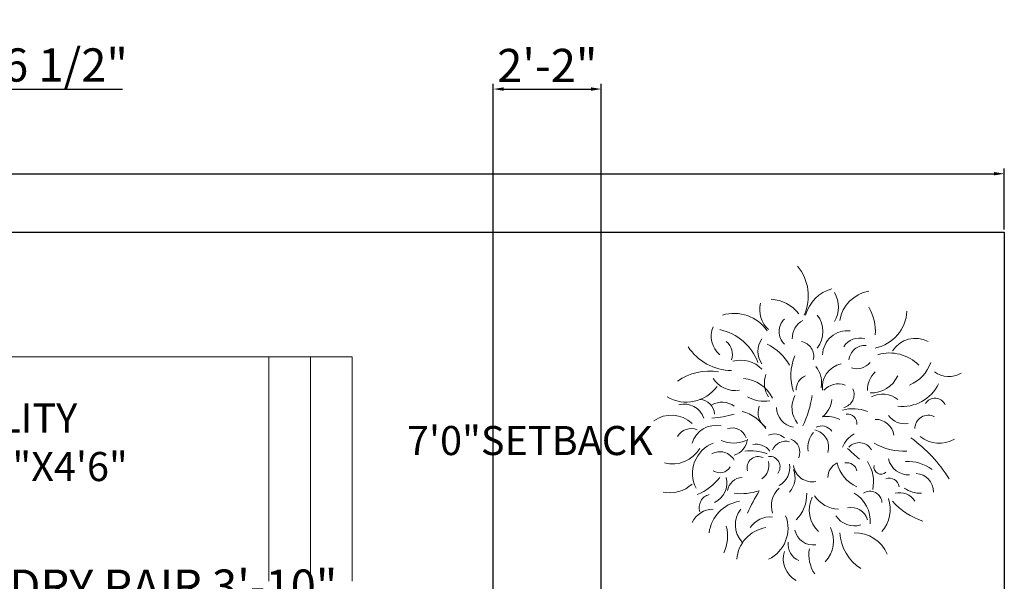
# Model space of a CAD drawing. Units: inches. Extents: x 3394 to 4794, y 965 to 1718.
# Tile 11 of 15: x 3704 to 3941, y 1583 to 1718. Entities that reach past the tile are written whole.
import ezdxf

# ---------------------------------------------------------------- set-up
doc = ezdxf.new("R2010")
doc.units = ezdxf.units.IN
for name, color, linetype, lineweight in [('A-ANNO-DIMS', 2, 'Continuous', 13), ('A-ANNO-TEXT', 7, 'Continuous', 18), ('A-AREA-IDEN', 7, 'Continuous', 18), ('A-FLOR', 7, 'Continuous', 18), ('A-FLOR-STRS', 7, 'Continuous', 18), ('C-PROP', 7, 'Continuous', 25), ('CAY', 94, 'Continuous', 13)]:
    doc.layers.add(name, color=color, linetype=linetype, lineweight=lineweight)
doc.styles.add('ATT', font='romans.shx')
doc.styles.get("Standard").update_dxf_attribs({"font": 'arial.ttf'})
doc.dimstyles.new('ISO-25', dxfattribs={"dimtxt": 8, "dimasz": 2.5, "dimexe": 1.25, "dimexo": 0.625, "dimtad": 1, "dimlunit": 3, "dimtxsty": 'Standard', "dimcen": 2.5, "dimadec": 0, "dimazin": 0, "dimtfac": 1, "dimtmove": 0, "dimatfit": 3, "dimfxl": 1, "dimarcsym": 0})

# ---------------------------------------------------------------- blocks, each defined once
blk = doc.blocks.new('12PPLT14')
at = {"color": 0, "linetype": 'ByBlock'}
for centre, radius, start, end in [((-0.1625, 0.4338), 0.1552, 335.4234, 39.9527), ((0.1087, 0.3325), 0.1308, 106.3737, 163.6865), ((-0.0015, 0.3959), 0.0956, 329.2952, 30.7048), ((0.216, 0.3316), 0.1193, 99.6686, 170.3916), ((-0.0808, 0.3868), 0.0897, 165.5676, 227.7978), ((-0.1402, 0.294), 0.1288, 38.2331, 86.4254), ((-0.2571, 0.2399), 0.1351, 34.2662, 106.816), ((-0.0514, 0.3138), 0.0928, 323.3029, 36.6971), ((0.0506, 0.3121), 0.1678, 356.7873, 29.9706), ((0.1909, 0.3893), 0.1338, 281.7312, 357.1257), ((-0.0467, 0.3138), 0.0589, 134.2792, 225.7208), ((0.0083, 0.2908), 0.0696, 119.3333, 181.2289), ((-0.2523, 0.2979), 0.0813, 157.2527, 229.5051), ((-0.3428, 0.1468), 0.1777, 20.6522, 77.761), ((0.1238, 0.2336), 0.083, 82.9962, 178.2659), ((-0.3207, 0.2361), 0.0583, 342.2672, 49.5918), ((-0.1032, 0.2472), 0.0733, 144.9004, 215.0996), ((-0.223, 0.1138), 0.1758, 29.5718, 63.8395), ((-0.0403, 0.2301), 0.0513, 346.7243, 78.6914), ((0.1649, 0.2288), 0.0631, 73.677, 147.4747), ((0.1827, 0.2139), 0.0534, 85.265, 175.2671), ((0.3529, 0.1986), 0.0923, 62.4899, 146.6083), ((-0.2631, 0.3606), 0.1778, 213.4024, 269.326), ((0.2662, 0.1039), 0.1379, 44.5227, 106.5076), ((-0.2335, 0.1217), 0.0961, 42.9815, 106.4777), ((0.103, 0.1659), 0.1687, 157.0616, 198.7007), ((0.1187, 0.1278), 0.0788, 101.6359, 188.4366), ((0.1561, 0.2471), 0.0582, 252.2434, 319.6792), ((0.2843, 0.2512), 0.1271, 292.7233, 340.8083), ((-0.3406, -0.0039), 0.1849, 80.336, 125.1387), ((-0.071, 0.1405), 0.0841, 159.833, 213.5727), ((-0.0525, 0.1406), 0.0902, 350.0819, 37.9622), ((0.2797, 0.1152), 0.0882, 134.2975, 179.349), ((0.4652, 0.2401), 0.0779, 232.4069, 301.8623), ((-0.2521, 0.2046), 0.0894, 212.7771, 278.7223), ((-0.2353, 0.0367), 0.1199, 26.1776, 85.1926), ((0.002, 0.1188), 0.05, 112.1748, 182.9374), ((0.094, 0.072), 0.0659, 70.3325, 137.7683), ((0.2042, 0.2053), 0.098, 267.7941, 335.7788), ((0.3092, 0.1973), 0.1353, 263.3454, 334.185), ((-0.4178, 0.2048), 0.1282, 239.7244, 324.0772), ((0.1017, 0.1024), 0.045, 282.8815, 24.0365), ((0.2424, 0.0217), 0.0815, 51.1397, 117.4271), ((-0.4247, -0.0009), 0.0706, 19.8329, 104.6003), ((-0.3739, 0.0341), 0.0511, 2.467, 87.4728), ((-0.2974, 0.0074), 0.0691, 53.5126, 119.7474), ((-0.1543, 0.2003), 0.1209, 241.5287, 278.4347), ((0.0228, 0.0586), 0.0851, 152.0419, 218.8274), ((-0.34, 0.1477), 0.3488, 334.29, 351.8885), ((-0.0111, 0.0925), 0.0832, 308.5351, 354.9136), ((0.4187, 0.0518), 0.0378, 24.3786, 147.9852), ((-0.3432, 0.3083), 0.2855, 272.3147, 287.7219), ((-0.2616, -0.0829), 0.132, 32.2356, 76.0319), ((-0.1183, 0.0408), 0.0581, 157.5609, 237.1128), ((-0.0447, 0.0607), 0.0698, 181.7454, 260.0237), ((0.1427, -0.0803), 0.1346, 68.7259, 105.2422), ((0.125, 0.0053), 0.0314, 351.8398, 98.1), ((-0.468, -0.0701), 0.1027, 47.2022, 124.8992), ((0.0563, -0.0634), 0.0921, 62.7918, 99.6978), ((0.2201, -0.0419), 0.0605, 6.851, 91.8869), ((0.3159, 0.0688), 0.0649, 214.6894, 281.6662), ((0.3966, -0.0128), 0.0455, 62.415, 179.5656), ((-0.4019, -0.0635), 0.0512, 65.2631, 151.643), ((-0.3178, -0.086), 0.0842, 78.2859, 162.9253), ((-0.2636, -0.0603), 0.0501, 19.5336, 107.2881), ((-0.1211, -0.079), 0.0486, 46.81, 114.2458), ((0.0687, -0.0762), 0.0776, 139.4669, 188.6741), ((0.0015, -0.0752), 0.0596, 343.1915, 77.687), ((0.0376, -0.0452), 0.0417, 34.8572, 117.0419), ((0.197, -0.1152), 0.0984, 120.3942, 155.6913), ((-0.2877, -0.1629), 0.109, 111.2663, 206.9249), ((-0.2585, 0.0428), 0.1041, 246.1369, 293.8631), ((-0.2726, -0.0426), 0.0609, 285.5398, 354.9083), ((-0.1835, -0.1238), 0.059, 37.3855, 100.4991), ((-0.0834, -0.1038), 0.0488, 74.167, 155.4291), ((-0.0828, -0.0921), 0.0473, 337.5706, 68.783), ((0.1639, -0.1068), 0.0471, 29.6516, 136.9148), ((0.3131, 0.1083), 0.1966, 239.6382, 273.343), ((0.055, -0.4368), 0.4844, 31.8508, 54.2708), ((0.4332, 0.0428), 0.1041, 231.8734, 299.32), ((-0.465, -0.0212), 0.1099, 256.1392, 328.2356), ((-0.3051, -0.1456), 0.0555, 28.564, 118.6243), ((-0.2031, -0.2618), 0.1748, 70.7416, 95.8247), ((0.3403, 0.1226), 0.295, 223.1416, 233.5315), ((-0.1751, -0.1446), 0.0382, 64.5989, 195.0715), ((-0.1983, -0.1346), 0.0584, 307.0043, 10.961), ((-0.1379, -0.1412), 0.0356, 321.496, 95.0552), ((-0.1367, -0.1434), 0.0675, 297.4603, 9.4578), ((0.1122, -0.1766), 0.0537, 114.9911, 180.121), ((0.2021, -0.1018), 0.1155, 193.035, 246.5169), ((0.1228, -0.1611), 0.0339, 11.252, 101.3122), ((0.0954, -0.19), 0.1169, 346.8331, 34.7134), ((0.3301, -0.0984), 0.0696, 193.4793, 272.7231), ((0.3295, -0.2531), 0.1299, 52.4116, 94.1568), ((-0.3049, -0.1199), 0.0412, 237.1862, 328.8294), ((-0.1261, -0.1768), 0.0743, 318.9446, 21.0601), ((0.0056, -0.1284), 0.0629, 187.6037, 281.9043), ((0.2371, -0.1417), 0.0239, 167.9887, 313.8509), ((0.3525, -0.2241), 0.0608, 358.6144, 87.0834), ((-0.4582, -0.0549), 0.1957, 293.3946, 321.4742), ((-0.3545, -0.1945), 0.0737, 295.4172, 13.937), ((-0.2272, -0.2284), 0.0518, 92.735, 171.8723), ((0.265, -0.2125), 0.0333, 8.0854, 109.9339), ((-0.4721, -0.1203), 0.1079, 257.3279, 313.213), ((-0.2342, -0.0362), 0.1951, 263.4737, 288.5568), ((0.4875, -0.6182), 0.7699, 148.9497, 155.3056), ((-0.0491, -0.2722), 0.0823, 133.2929, 197.2496), ((-0.1342, -0.2328), 0.1218, 315.1067, 1.332), ((0.0948, -0.3222), 0.106, 354.6407, 60.4156), ((0.2004, -0.2632), 0.04, 3.1298, 123.6919), ((0.3002, -0.2876), 0.0597, 31.279, 105.0766), ((0.3711, -0.1347), 0.0953, 234.4297, 271.3309), ((-0.3303, -0.2772), 0.044, 103.5534, 199.8954), ((-0.2197, -0.3768), 0.1216, 98.9327, 173.5652), ((0.0958, -0.2858), 0.1, 154.8808, 226.8679), ((0.0984, -0.1813), 0.1021, 214.3427, 267.4969), ((0.1534, -0.2836), 0.1149, 319.1908, 18.2125), ((0.4504, -0.1006), 0.2342, 221.7868, 251.9354), ((-0.3258, -0.3645), 0.0813, 91.0528, 153.0122), ((-0.1666, -0.3361), 0.0858, 141.9374, 222.639), ((0.137, -0.3342), 0.0567, 15.8404, 102.1789), ((-0.1356, -0.3909), 0.0814, 84.4526, 145.9961), ((-0.1912, -0.3476), 0.1157, 295.6702, 21.368), ((0.1487, -0.2627), 0.0766, 213.8932, 285.618), ((-0.4022, -0.3739), 0.1237, 333.1557, 15.4351), ((-0.1321, -0.4596), 0.1156, 98.8586, 176.1805), ((0.0095, -0.3403), 0.0634, 192.7121, 278.2146), ((-0.0287, -0.3897), 0.1058, 317.7735, 24.7522), ((0.2528, -0.3527), 0.1547, 183.8744, 237.3741), ((0.1506, -0.4799), 0.1168, 23.0406, 91.6662), ((-0.0165, -0.4023), 0.0586, 172.0702, 247.3677), ((-0.0081, -0.4497), 0.0833, 162.968, 241.4878), ((0.1108, -0.4364), 0.1161, 170.0959, 213.6572)]:
    blk.add_arc(centre, radius, start, end, dxfattribs=at)
at = {"color": 0, "linetype": 'ByBlock', "style": 'ATT'}
for tag, p, flags in [('ITEM', (-1.4111, -3.0457), 3), ('ROOM_NUMBER', (-1.4111, -4.379), 1)]:
    blk.add_attdef(tag, p, '', height=1, dxfattribs=dict(at, flags=flags))
blk = doc.blocks.new('*D30')
at = {"layer": 'A-ANNO-DIMS', "color": 0, "lineweight": -2, "transparency": 16777216}
for p, q in [((3427.74, 1667.31), (3427.74, 1682.01)), ((3430.24, 1680.76), (3938.24, 1680.76)), ((3940.74, 1667.31), (3940.74, 1682.01))]:
    blk.add_line(p, q, dxfattribs=at)
at = {"layer": 'A-ANNO-DIMS', "color": 0, "transparency": 16777216}
for points in [[(3430.24, 1681.18), (3430.24, 1680.35), (3427.74, 1680.76)], [(3938.24, 1681.18), (3938.24, 1680.35), (3940.74, 1680.76)]]:
    blk.add_solid(points, dxfattribs=at)
at = {"layer": 'Defpoints', "color": 0, "transparency": 16777216}
for p in [(3940.74, 1680.76), (3427.74, 1666.68), (3940.74, 1666.68)]:
    blk.add_point(p, dxfattribs=at)
at = {"layer": 'A-ANNO-DIMS', "color": 0, "transparency": 16777216, "insert": (3684.24, 1685.47), "char_height": 8, "attachment_point": 5}
blk.add_mtext('42\'-9"', dxfattribs=at)
blk = doc.blocks.new('*D92')
at = {"layer": 'A-ANNO-DIMS', "color": 0, "lineweight": -2, "transparency": 16777216}
for p, q in [((3620.92, 1582.06), (3620.92, 1574.52)), ((3667.02, 1582.06), (3667.02, 1574.52)), ((3623.42, 1575.77), (3664.52, 1575.77)), ((3667.02, 1575.77), (3783.6, 1575.77))]:
    blk.add_line(p, q, dxfattribs=at)
at = {"layer": 'A-ANNO-DIMS', "color": 0, "transparency": 16777216}
for points in [[(3623.42, 1576.18), (3623.42, 1575.35), (3620.92, 1575.77)], [(3664.52, 1576.18), (3664.52, 1575.35), (3667.02, 1575.77)]]:
    blk.add_solid(points, dxfattribs=at)
at = {"layer": 'Defpoints', "color": 0, "transparency": 16777216}
for p in [(3620.92, 1582.68), (3667.02, 1582.68), (3667.02, 1575.77)]:
    blk.add_point(p, dxfattribs=at)
at = {"layer": 'A-ANNO-DIMS', "color": 0, "transparency": 16777216, "insert": (3726.56, 1580.48), "char_height": 8, "attachment_point": 5}
blk.add_mtext('LAUNDRY PAIR 3\'-10"', dxfattribs=at)
blk = doc.blocks.new('*D124')
at = {"layer": 'A-ANNO-DIMS', "color": 0, "lineweight": -2, "transparency": 16777216}
for p, q in [((3667.02, 1583.31), (3667.02, 1702.38)), ((3685.62, 1583.31), (3685.62, 1702.38)), ((3669.52, 1701.13), (3683.12, 1701.13)), ((3685.62, 1701.13), (3728.52, 1701.13))]:
    blk.add_line(p, q, dxfattribs=at)
at = {"layer": 'A-ANNO-DIMS', "color": 0, "transparency": 16777216}
for points in [[(3669.52, 1701.55), (3669.52, 1700.72), (3667.02, 1701.13)], [(3683.12, 1701.55), (3683.12, 1700.72), (3685.62, 1701.13)]]:
    blk.add_solid(points, dxfattribs=at)
at = {"layer": 'Defpoints', "color": 0, "transparency": 16777216}
for p in [(3685.62, 1701.13), (3667.02, 1582.68), (3685.62, 1582.68)]:
    blk.add_point(p, dxfattribs=at)
at = {"layer": 'A-ANNO-DIMS', "color": 0, "transparency": 16777216, "insert": (3708.32, 1705.89), "char_height": 8, "attachment_point": 5}
blk.add_mtext('1\'-6 1/2"', dxfattribs=at)
blk = doc.blocks.new('*D126')
at = {"layer": 'A-ANNO-DIMS', "color": 0, "lineweight": -2, "transparency": 16777216}
for p, q in [((3817.74, 1382.31), (3817.74, 1702.38)), ((3843.73, 1380.81), (3843.73, 1702.38)), ((3820.24, 1701.13), (3841.23, 1701.13))]:
    blk.add_line(p, q, dxfattribs=at)
at = {"layer": 'A-ANNO-DIMS', "color": 0, "transparency": 16777216}
for points in [[(3820.24, 1701.55), (3820.24, 1700.72), (3817.74, 1701.13)], [(3841.23, 1701.55), (3841.23, 1700.72), (3843.73, 1701.13)]]:
    blk.add_solid(points, dxfattribs=at)
at = {"layer": 'Defpoints', "color": 0, "transparency": 16777216}
for p in [(3843.73, 1701.13), (3817.74, 1381.68), (3843.73, 1380.18)]:
    blk.add_point(p, dxfattribs=at)
at = {"layer": 'A-ANNO-DIMS', "color": 0, "transparency": 16777216, "insert": (3830.74, 1705.77), "char_height": 8, "attachment_point": 5}
blk.add_mtext('2\'-2"', dxfattribs=at)

msp = doc.modelspace()

# ---------------------------------------------------------------- linework, layer by layer
at = {"layer": 'A-FLOR'}
msp.add_line((3783.745, 1636.682), (3604.745, 1636.682), dxfattribs=at)
at = {"layer": 'A-FLOR-STRS'}
for p, q in [((3763.745, 1582.682), (3763.745, 1636.682)), ((3773.745, 1582.682), (3773.745, 1636.682)), ((3783.745, 1582.682), (3783.745, 1636.682))]:
    msp.add_line(p, q, dxfattribs=at)
at = {"layer": 'C-PROP'}
for p, q in [((3427.745, 1666.682), (3940.745, 1666.682)), ((3940.745, 1666.682), (3940.745, 1057.682))]:
    msp.add_line(p, q, dxfattribs=at)

# ---------------------------------------------------------------- block references
at = {"layer": 'CAY', "xscale": 71.57720376410516, "yscale": 71.57720376410516, "zscale": 71.57720376410516}
msp.add_blockref('12PPLT14', (3894.085, 1620.317), dxfattribs=at)

# ---------------------------------------------------------------- texts
at = {"layer": 'A-ANNO-TEXT', "insert": (3796.969, 1620.056), "char_height": 7, "attachment_point": 1}
msp.add_mtext_dynamic_manual_height_columns('{\\fTimes New Roman|b0|i0|c0|p18;7\'0"SETBACK}', width=61.05572, gutter_width=12.5, heights=[0], dxfattribs=at)
at = {"layer": 'A-AREA-IDEN', "insert": (3683.427, 1625.469), "char_height": 7, "attachment_point": 1}
msp.add_mtext_dynamic_manual_height_columns('{\\fTimes New Roman|b0|i0|c0|p18;UTILITY\\P13\'3"X4\'6"}', width=61.05572, gutter_width=12.5, heights=[0], dxfattribs=at)

# ---------------------------------------------------------------- dimensions: what is measured, and where the dimension line sits
at = {"layer": 'A-ANNO-DIMS'}
for base, p1, p2, override, picture, middle in [((3685.617, 1701.132), (3667.022, 1582.682), (3685.617, 1582.682), {"dimdec": 1, "dimlfac": 1, "dimrnd": 0, "dimzin": 1, "dimdsep": 46, "dimlunit": 4, "dimfrac": 2}, '*D124', (3708.319, 1705.894)), ((3843.735, 1701.132), (3817.745, 1381.682), (3843.735, 1380.182), {"dimdec": 1, "dimlfac": 1, "dimrnd": 0, "dimzin": 1, "dimdsep": 46, "dimlunit": 4, "dimfrac": 2}, '*D126', (3830.74, 1705.774)), ((3940.745, 1680.764), (3427.745, 1666.682), (3940.745, 1666.682), {"dimclrd": 0, "dimclre": 0, "dimclrt": 0}, '*D30', (3684.245, 1685.474))]:
    dim = msp.add_linear_dim(base=base, p1=p1, p2=p2, dimstyle='ISO-25', override=override, dxfattribs=at)
    dim.commit()
    dim.dimension.update_dxf_attribs({"geometry": picture, "text_midpoint": middle})
dim = msp.add_linear_dim(base=(3667.022, 1575.767), p1=(3620.921, 1582.682), p2=(3667.022, 1582.682), text='LAUNDRY PAIR <>', dimstyle='ISO-25', override={"dimdec": 1, "dimlfac": 1, "dimrnd": 0, "dimzin": 1, "dimdsep": 46, "dimlunit": 4, "dimfrac": 2}, dxfattribs=at)
dim.commit()
dim.dimension.update_dxf_attribs({"geometry": '*D92', "text_midpoint": (3726.561, 1580.48)})

doc.saveas('drawing.dxf')
